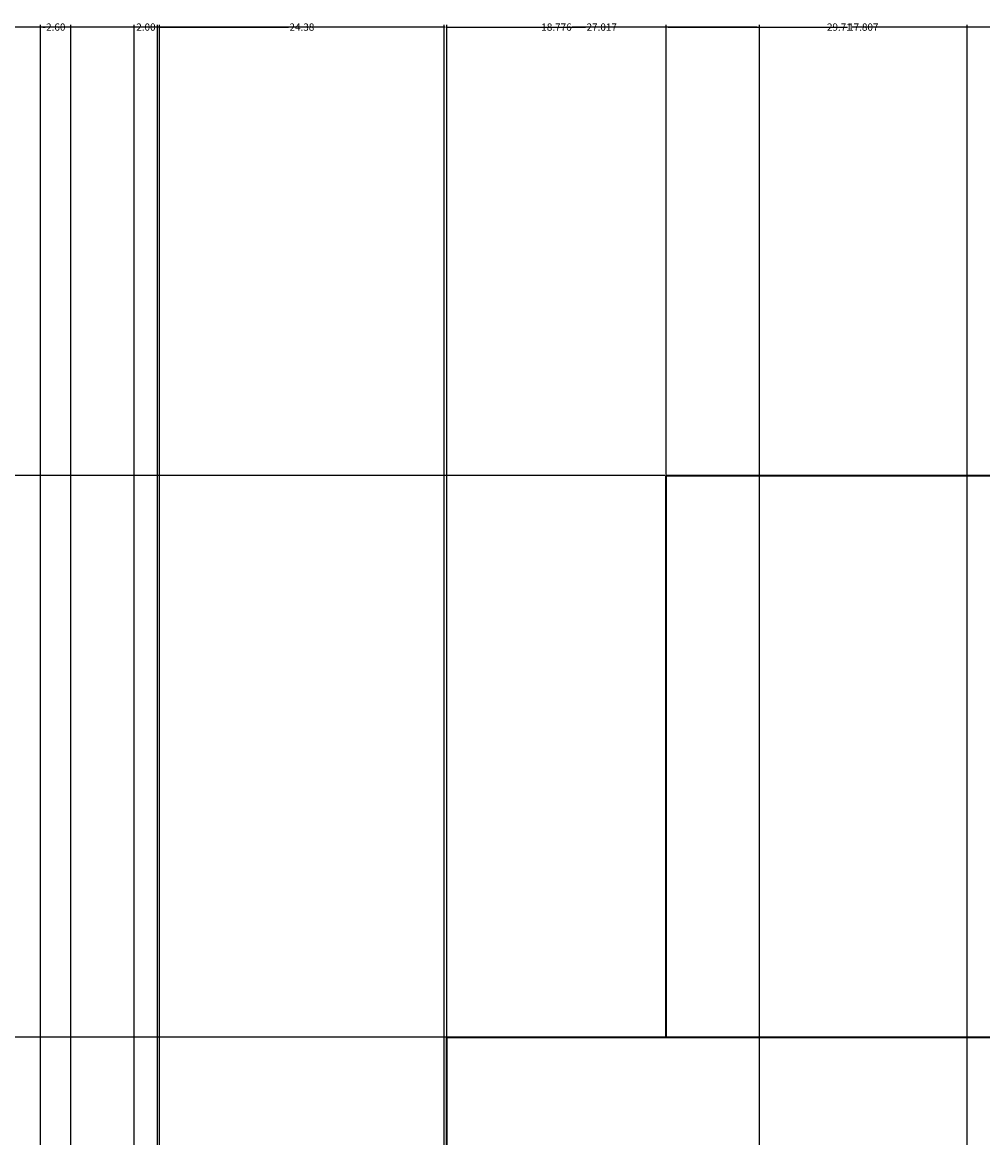
# Model space of a CAD drawing. Units: inches. Extents: x -13 to 809, y 112 to 656.
# Tile 35 of 55: x 257 to 339, y 561 to 656. Entities that reach past the tile are written whole.
import ezdxf

# ---------------------------------------------------------------- set-up
doc = ezdxf.new("R2010")
doc.units = ezdxf.units.IN
doc.header["$MEASUREMENT"] = 0
doc.layers.add('A-ANNO-DIMS', color=2, linetype='Continuous', lineweight=18)
doc.layers.add('A-ELEV', color=7, linetype='Continuous', lineweight=35)
doc.styles.get("Standard").update_dxf_attribs({"font": 'arial.ttf'})
doc.dimstyles.get("Standard").update_dxf_attribs({"dimtxt": 0.625, "dimasz": 0.18, "dimexe": 0.18, "dimexo": 0.0625, "dimgap": 0.09, "dimtad": 0, "dimtih": 1, "dimtoh": 1, "dimdec": 4, "dimzin": 0, "dimdsep": 46, "dimlunit": 4, "dimtxsty": 'Standard', "dimcen": 0.09, "dimadec": 0, "dimazin": 0, "dimtfac": 1, "dimtdec": 4, "dimtofl": 0, "dimtmove": 0, "dimatfit": 3, "dimfxl": 1, "dimtolj": 1, "dimtzin": 0, "dimarcsym": 0})

# ---------------------------------------------------------------- blocks, each defined once
blk = doc.blocks.new('*D23')
at = {"layer": 'A-ANNO-DIMS', "color": 0, "lineweight": -2, "transparency": 16777216}
for p, q in [((107.259, 510.582), (107.259, 655.963)), ((107.439, 655.783), (198.733, 655.783)), ((292.743, 655.783), (201.449, 655.783)), ((292.923, 569.304), (292.923, 655.963))]:
    blk.add_line(p, q, dxfattribs=at)
at = {"layer": 'A-ANNO-DIMS', "color": 0, "transparency": 16777216}
for points in [[(107.439, 655.813), (107.439, 655.753), (107.259, 655.783)], [(292.743, 655.813), (292.743, 655.753), (292.923, 655.783)]]:
    blk.add_solid(points, dxfattribs=at)
at = {"layer": 'Defpoints', "color": 0, "transparency": 16777216}
for p in [(292.923, 655.783), (292.923, 569.241), (107.259, 510.52)]:
    blk.add_point(p, dxfattribs=at)
at = {"layer": 'A-ANNO-DIMS', "color": 0, "transparency": 16777216, "insert": (200.091, 655.783), "char_height": 0.625, "attachment_point": 5}
blk.add_mtext('\\A1;185.66', dxfattribs=at)
blk = doc.blocks.new('*D24')
at = {"layer": 'A-ANNO-DIMS', "color": 0, "lineweight": -2, "transparency": 16777216}
for p, q in [((292.923, 569.304), (292.923, 655.963)), ((293.103, 655.783), (300.953, 655.783)), ((311.519, 655.783), (303.669, 655.783)), ((311.699, 617.433), (311.699, 655.963))]:
    blk.add_line(p, q, dxfattribs=at)
at = {"layer": 'A-ANNO-DIMS', "color": 0, "transparency": 16777216}
for points in [[(293.103, 655.813), (293.103, 655.753), (292.923, 655.783)], [(311.519, 655.813), (311.519, 655.753), (311.699, 655.783)]]:
    blk.add_solid(points, dxfattribs=at)
at = {"layer": 'Defpoints', "color": 0, "transparency": 16777216}
for p in [(311.699, 655.783), (311.699, 617.371), (292.923, 569.241)]:
    blk.add_point(p, dxfattribs=at)
at = {"layer": 'A-ANNO-DIMS', "color": 0, "transparency": 16777216, "insert": (302.311, 655.783), "char_height": 0.625, "attachment_point": 5}
blk.add_mtext('\\A1;18.776', dxfattribs=at)
blk = doc.blocks.new('*D25')
at = {"layer": 'A-ANNO-DIMS', "color": 0, "lineweight": -2, "transparency": 16777216}
for p, q in [((311.699, 617.433), (311.699, 655.963)), ((311.879, 655.783), (325.464, 655.783)), ((341.227, 655.783), (327.643, 655.783)), ((341.407, 524.343), (341.407, 655.963))]:
    blk.add_line(p, q, dxfattribs=at)
at = {"layer": 'A-ANNO-DIMS', "color": 0, "transparency": 16777216}
for points in [[(311.879, 655.813), (311.879, 655.753), (311.699, 655.783)], [(341.227, 655.813), (341.227, 655.753), (341.407, 655.783)]]:
    blk.add_solid(points, dxfattribs=at)
at = {"layer": 'Defpoints', "color": 0, "transparency": 16777216}
for p in [(341.407, 655.783), (311.699, 617.371), (341.407, 524.281)]:
    blk.add_point(p, dxfattribs=at)
at = {"layer": 'A-ANNO-DIMS', "color": 0, "transparency": 16777216, "insert": (326.553, 655.783), "char_height": 0.625, "attachment_point": 5}
blk.add_mtext('\\A1;29.71', dxfattribs=at)
blk = doc.blocks.new('*D36')
at = {"layer": 'A-ANNO-DIMS', "color": 0, "lineweight": -2, "transparency": 16777216}
for p, q in [((311.637, 569.241), (-12.099, 569.241)), ((-11.919, 569.061), (-11.919, 540.29)), ((-11.919, 510.7), (-11.919, 539.472)), ((107.196, 510.52), (-12.099, 510.52))]:
    blk.add_line(p, q, dxfattribs=at)
at = {"layer": 'A-ANNO-DIMS', "color": 0, "transparency": 16777216}
for points in [[(-11.949, 569.061), (-11.889, 569.061), (-11.919, 569.241)], [(-11.949, 510.7), (-11.889, 510.7), (-11.919, 510.52)]]:
    blk.add_solid(points, dxfattribs=at)
at = {"layer": 'Defpoints', "color": 0, "transparency": 16777216}
for p in [(-11.919, 569.241), (311.699, 569.241), (107.259, 510.52)]:
    blk.add_point(p, dxfattribs=at)
at = {"layer": 'A-ANNO-DIMS', "color": 0, "transparency": 16777216, "insert": (-11.919, 539.881), "char_height": 0.625, "attachment_point": 5}
blk.add_mtext('\\A1;58.72', dxfattribs=at)
blk = doc.blocks.new('*D37')
at = {"layer": 'A-ANNO-DIMS', "color": 0, "lineweight": -2, "transparency": 16777216}
for p, q in [((311.637, 617.371), (-12.099, 617.371)), ((-11.919, 617.191), (-11.919, 593.715)), ((-11.919, 569.421), (-11.919, 592.897)), ((311.637, 569.241), (-12.099, 569.241))]:
    blk.add_line(p, q, dxfattribs=at)
at = {"layer": 'A-ANNO-DIMS', "color": 0, "transparency": 16777216}
for points in [[(-11.949, 617.191), (-11.889, 617.191), (-11.919, 617.371)], [(-11.949, 569.421), (-11.889, 569.421), (-11.919, 569.241)]]:
    blk.add_solid(points, dxfattribs=at)
at = {"layer": 'Defpoints', "color": 0, "transparency": 16777216}
for p in [(-11.919, 617.371), (311.699, 617.371), (311.699, 569.241)]:
    blk.add_point(p, dxfattribs=at)
at = {"layer": 'A-ANNO-DIMS', "color": 0, "transparency": 16777216, "insert": (-11.919, 593.306), "char_height": 0.625, "attachment_point": 5}
blk.add_mtext('\\A1;48.13', dxfattribs=at)
blk = doc.blocks.new('*D100')
at = {"layer": 'A-ANNO-DIMS', "color": 0, "lineweight": -2, "transparency": 16777216}
for p, q in [((239.308, 452.625), (239.308, 655.963)), ((239.488, 655.783), (252.413, 655.783)), ((268.122, 655.783), (255.196, 655.783)), ((268.302, 452.625), (268.302, 655.963))]:
    blk.add_line(p, q, dxfattribs=at)
at = {"layer": 'A-ANNO-DIMS', "color": 0, "transparency": 16777216}
for points in [[(239.488, 655.813), (239.488, 655.753), (239.308, 655.783)], [(268.122, 655.813), (268.122, 655.753), (268.302, 655.783)]]:
    blk.add_solid(points, dxfattribs=at)
at = {"layer": 'Defpoints', "color": 0, "transparency": 16777216}
for p in [(268.302, 655.783), (239.308, 452.563), (268.302, 452.563)]:
    blk.add_point(p, dxfattribs=at)
at = {"layer": 'A-ANNO-DIMS', "color": 0, "transparency": 16777216, "insert": (253.805, 655.783), "char_height": 0.625, "attachment_point": 5}
blk.add_mtext('\\A1;28.994', dxfattribs=at)
blk = doc.blocks.new('*D101')
at = {"layer": 'A-ANNO-DIMS', "color": 0, "lineweight": -2, "transparency": 16777216}
for p, q in [((268.302, 452.625), (268.302, 655.963)), ((268.482, 655.783), (279.342, 655.783)), ((292.503, 655.783), (281.643, 655.783)), ((292.683, 452.625), (292.683, 655.963))]:
    blk.add_line(p, q, dxfattribs=at)
at = {"layer": 'A-ANNO-DIMS', "color": 0, "transparency": 16777216}
for points in [[(268.482, 655.813), (268.482, 655.753), (268.302, 655.783)], [(292.503, 655.813), (292.503, 655.753), (292.683, 655.783)]]:
    blk.add_solid(points, dxfattribs=at)
at = {"layer": 'Defpoints', "color": 0, "transparency": 16777216}
for p in [(292.683, 655.783), (268.302, 452.563), (292.683, 452.563)]:
    blk.add_point(p, dxfattribs=at)
at = {"layer": 'A-ANNO-DIMS', "color": 0, "transparency": 16777216, "insert": (280.493, 655.783), "char_height": 0.625, "attachment_point": 5}
blk.add_mtext('\\A1;24.38', dxfattribs=at)
blk = doc.blocks.new('*D102')
at = {"layer": 'A-ANNO-DIMS', "color": 0, "lineweight": -2, "transparency": 16777216}
for p, q in [((292.683, 452.625), (292.683, 655.963)), ((292.863, 655.783), (304.799, 655.783)), ((319.52, 655.783), (307.584, 655.783)), ((319.7, 452.625), (319.7, 655.963))]:
    blk.add_line(p, q, dxfattribs=at)
at = {"layer": 'A-ANNO-DIMS', "color": 0, "transparency": 16777216}
for points in [[(292.863, 655.813), (292.863, 655.753), (292.683, 655.783)], [(319.52, 655.813), (319.52, 655.753), (319.7, 655.783)]]:
    blk.add_solid(points, dxfattribs=at)
at = {"layer": 'Defpoints', "color": 0, "transparency": 16777216}
for p in [(319.7, 655.783), (292.683, 452.563), (319.7, 452.563)]:
    blk.add_point(p, dxfattribs=at)
at = {"layer": 'A-ANNO-DIMS', "color": 0, "transparency": 16777216, "insert": (306.192, 655.783), "char_height": 0.625, "attachment_point": 5}
blk.add_mtext('\\A1;27.017', dxfattribs=at)
blk = doc.blocks.new('*D103')
at = {"layer": 'A-ANNO-DIMS', "color": 0, "lineweight": -2, "transparency": 16777216}
for p, q in [((319.7, 452.625), (319.7, 655.963)), ((319.88, 655.783), (327.246, 655.783)), ((337.327, 655.783), (329.962, 655.783)), ((337.507, 462.582), (337.507, 655.963))]:
    blk.add_line(p, q, dxfattribs=at)
at = {"layer": 'A-ANNO-DIMS', "color": 0, "transparency": 16777216}
for points in [[(319.88, 655.813), (319.88, 655.753), (319.7, 655.783)], [(337.327, 655.813), (337.327, 655.753), (337.507, 655.783)]]:
    blk.add_solid(points, dxfattribs=at)
at = {"layer": 'Defpoints', "color": 0, "transparency": 16777216}
for p in [(337.507, 655.783), (337.507, 462.52), (319.7, 452.563)]:
    blk.add_point(p, dxfattribs=at)
at = {"layer": 'A-ANNO-DIMS', "color": 0, "transparency": 16777216, "insert": (328.604, 655.783), "char_height": 0.625, "attachment_point": 5}
blk.add_mtext('\\A1;17.807', dxfattribs=at)
blk = doc.blocks.new('*D116')
at = {"layer": 'A-ANNO-DIMS', "color": 0, "lineweight": -2, "transparency": 16777216}
for p, q in [((258.102, 210.847), (258.102, 655.963)), ((258.282, 655.783), (258.497, 655.783)), ((260.525, 655.783), (260.309, 655.783)), ((260.705, 207.435), (260.705, 655.963))]:
    blk.add_line(p, q, dxfattribs=at)
at = {"layer": 'A-ANNO-DIMS', "color": 0, "transparency": 16777216}
for points in [[(258.282, 655.813), (258.282, 655.753), (258.102, 655.783)], [(260.525, 655.813), (260.525, 655.753), (260.705, 655.783)]]:
    blk.add_solid(points, dxfattribs=at)
at = {"layer": 'Defpoints', "color": 0, "transparency": 16777216}
for p in [(260.705, 655.783), (258.102, 210.785), (260.705, 207.372)]:
    blk.add_point(p, dxfattribs=at)
at = {"layer": 'A-ANNO-DIMS', "color": 0, "transparency": 16777216, "insert": (259.403, 655.783), "char_height": 0.625, "attachment_point": 5}
blk.add_mtext('\\A1;2.60', dxfattribs=at)
blk = doc.blocks.new('*D119')
at = {"layer": 'A-ANNO-DIMS', "color": 0, "lineweight": -2, "transparency": 16777216}
for p, q in [((265.9486, 655.782835), (265.7686, 655.782835)), ((266.1286, 207.43492), (266.1286, 655.962835)), ((268.1286, 207.43492), (268.1286, 655.962835)), ((268.3086, 655.782835), (268.4886, 655.782835))]:
    blk.add_line(p, q, dxfattribs=at)
at = {"layer": 'A-ANNO-DIMS', "color": 0, "transparency": 16777216}
for points in [[(265.9486, 655.812835), (265.9486, 655.752835), (266.1286, 655.782835)], [(268.3086, 655.812835), (268.3086, 655.752835), (268.1286, 655.782835)]]:
    blk.add_solid(points, dxfattribs=at)
at = {"layer": 'Defpoints', "color": 0, "transparency": 16777216}
for p in [(268.1286, 655.782835), (266.1286, 207.37242), (268.1286, 207.37242)]:
    blk.add_point(p, dxfattribs=at)
at = {"layer": 'A-ANNO-DIMS', "color": 0, "transparency": 16777216, "insert": (267.1286, 655.782835), "char_height": 0.625, "attachment_point": 5}
blk.add_mtext('\\A1;2.00', dxfattribs=at)

msp = doc.modelspace()

# ---------------------------------------------------------------- linework, layer by layer
at = {"layer": 'A-ELEV'}
for p, q in [((311.6991, 569.2414), (311.6991, 617.3708)), ((311.6991, 617.3708), (621.008, 617.3708)), ((292.923, 558.5199), (292.923, 569.2414)), ((292.923, 569.2414), (644.6221, 569.2414))]:
    msp.add_line(p, q, dxfattribs=at)

# ---------------------------------------------------------------- dimensions: what is measured, and where the dimension line sits
at = {"layer": 'A-ANNO-DIMS'}
for base, p1, p2, override, picture, middle in [((292.923, 655.7828), (107.2588, 510.5199), (292.923, 569.2414), {"dimdec": 2, "dimlfac": 1, "dimrnd": 0, "dimzin": 0, "dimdsep": 46, "dimlunit": 2}, '*D23', (200.0909, 655.7828)), ((268.3019, 655.7828), (239.3079, 452.5629), (268.3019, 452.5629), {"dimdec": 3, "dimlfac": 1, "dimrnd": 0, "dimzin": 0, "dimdsep": 46, "dimlunit": 2}, '*D100', (253.8049, 655.7828)), ((260.7048, 655.7828), (258.1022, 210.7849), (260.7048, 207.3724), {"dimdec": 2, "dimlfac": 1, "dimrnd": 0, "dimzin": 0, "dimdsep": 46, "dimlunit": 2}, '*D116', (259.4035, 655.7828)), ((268.1286, 655.7828), (266.1286, 207.3724), (268.1286, 207.3724), {"dimdec": 2, "dimlfac": 1, "dimrnd": 0, "dimzin": 0, "dimdsep": 46, "dimlunit": 2}, '*D119', (267.1286, 655.7828)), ((292.6832, 655.7828), (268.3019, 452.5629), (292.6832, 452.5629), {"dimdec": 2, "dimlfac": 1, "dimrnd": 0, "dimzin": 0, "dimdsep": 46, "dimlunit": 2}, '*D101', (280.4925, 655.7828)), ((319.7004, 655.7828), (292.6832, 452.5629), (319.7004, 452.5629), {"dimdec": 3, "dimlfac": 1, "dimrnd": 0, "dimzin": 0, "dimdsep": 46, "dimlunit": 2}, '*D102', (306.1918, 655.7828)), ((311.6991, 655.7828), (292.923, 569.2414), (311.6991, 617.3708), {"dimdec": 3, "dimlfac": 1, "dimrnd": 0, "dimzin": 0, "dimdsep": 46, "dimlunit": 2}, '*D24', (302.311, 655.7828)), ((341.4072, 655.7828), (311.6991, 617.3708), (341.4072, 524.281), {"dimdec": 2, "dimlfac": 1, "dimrnd": 0, "dimzin": 0, "dimdsep": 46, "dimlunit": 2}, '*D25', (326.5531, 655.7828)), ((337.5074, 655.7828), (319.7004, 452.5629), (337.5074, 462.5199), {"dimdec": 3, "dimlfac": 1, "dimrnd": 0, "dimzin": 0, "dimdsep": 46, "dimlunit": 2}, '*D103', (328.6039, 655.7828))]:
    dim = msp.add_linear_dim(base=base, p1=p1, p2=p2, dimstyle='Standard', override=override, dxfattribs=at)
    dim.commit()
    dim.dimension.update_dxf_attribs({"geometry": picture, "text_midpoint": middle})
for base, p1, p2, picture, middle in [((-11.9191, 617.3708), (311.6991, 569.2414), (311.6991, 617.3708), '*D37', (-11.9191, 593.3061)), ((-11.9191, 569.2414), (107.2588, 510.5199), (311.6991, 569.2414), '*D36', (-11.9191, 539.8806))]:
    dim = msp.add_linear_dim(base=base, p1=p1, p2=p2, angle=90, dimstyle='Standard', override={"dimdec": 2, "dimlfac": 1, "dimrnd": 0, "dimzin": 0, "dimdsep": 46, "dimlunit": 2}, dxfattribs=at)
    dim.commit()
    dim.dimension.update_dxf_attribs({"geometry": picture, "text_midpoint": middle})

doc.saveas('drawing.dxf')
